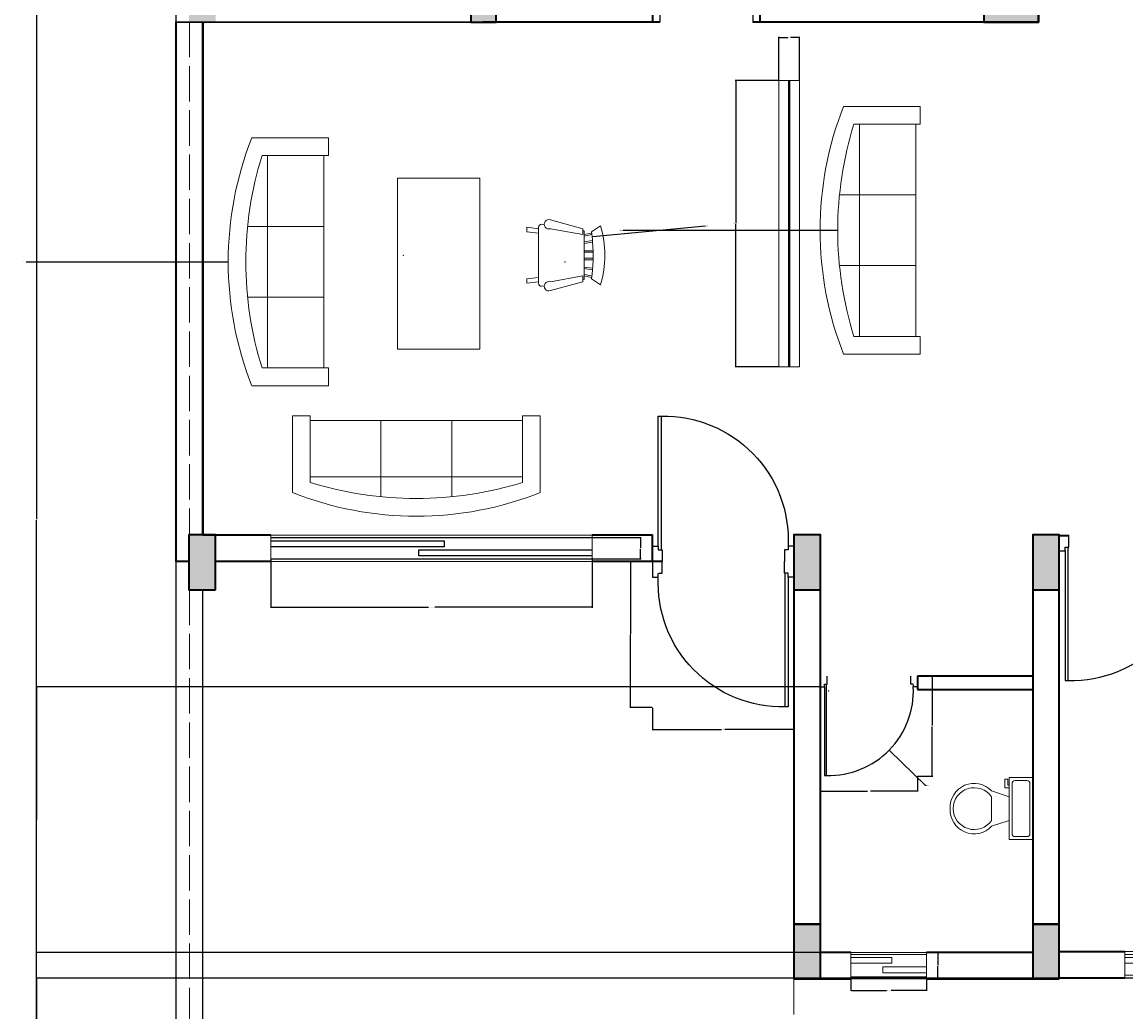
# Model space of a CAD drawing. Units: inches. Extents: x 2711 to 4246, y 540 to 1583.
# Tile 2 of 7: x 2711 to 3086, y 894 to 1230. Entities that reach past the tile are written whole.
import ezdxf

# ---------------------------------------------------------------- set-up
doc = ezdxf.new("R2010")
doc.units = ezdxf.units.IN
doc.linetypes.add('ACAD_ISO02W100', pattern=[15, 12, -3])
for name, color, linetype, lineweight in [('A-ANNO-DIMS', 2, 'Continuous', 18), ('A-COLS', 210, 'Continuous', 35), ('A-COLS-PATT', 6, 'Continuous', 13), ('A-FLOR-FIXT', 112, 'Continuous', 18), ('A-FLOR-OVHD', 225, 'ACAD_ISO02W100', 13), ('A-GLAZ', 4, 'Continuous', 18), ('A-WALL', 1, 'Continuous', 35), ('C-PROP-HIDN', 7, 'ACAD_ISO02W100', 13), ('C-PROP-WALL', 7, 'Continuous', 25), ('DOOR', 32, 'Continuous', 25), ('FURN', 30, 'Continuous', 18)]:
    doc.layers.add(name, color=color, linetype=linetype, lineweight=lineweight)
doc.layers.add('DARK', color=5, linetype='Continuous')
doc.styles.get("Standard").update_dxf_attribs({"font": 'arial.ttf'})
doc.dimstyles.get("Standard").update_dxf_attribs({"dimtxt": 0.18, "dimasz": 0.18, "dimexe": 0.18, "dimexo": 0.0625, "dimgap": 0.09, "dimtad": 0, "dimtih": 1, "dimtoh": 1, "dimdec": 4, "dimzin": 0, "dimdsep": 46, "dimtxsty": 'Standard', "dimcen": 0.09, "dimadec": 0, "dimazin": 0, "dimtfac": 1, "dimtdec": 4, "dimtofl": 0, "dimtmove": 0, "dimatfit": 3, "dimfxl": 1, "dimtolj": 1, "dimtzin": 0, "dimarcsym": 0})

# ---------------------------------------------------------------- blocks, each defined once
blk = doc.blocks.new('DOORS')
at = {"layer": 'DOOR'}
for p, q in [((-0.63, -0.36), (-0.63, -5.61)), ((2.62, -4.36), (2.62, -0.36)), ((44.12, -4.36), (44.12, -0.36)), ((47.37, -0.36), (47.37, -5.61)), ((-0.63, -5.61), (1.37, -5.61)), ((1.37, -5.61), (1.37, -4.36)), ((1.37, -4.36), (2.62, -4.36)), ((1.37, -5.61), (1.37, -49.61)), ((2.37, -49.61), (2.37, -4.36)), ((45.37, -4.36), (44.12, -4.36)), ((47.37, -5.61), (45.37, -5.61)), ((1.37, -49.61), (2.37, -49.61))]:
    blk.add_line(p, q, dxfattribs=at)
for centre, radius, start, end in [((3.41, -7.61), 42.01, 268.5852, 2.7319), ((38.76, -4.99), 6.64, 354.6023, 5.3977)]:
    blk.add_arc(centre, radius, start, end, dxfattribs=at)
blk = doc.blocks.new('DIPDASS')
at = {"layer": 'DARK'}
for p, q in [((0, 0), (109.02, 0)), ((0, -7.25), (109.02, -7.25))]:
    blk.add_line(p, q, dxfattribs=at)
at = {"layer": 'DOOR'}
for points in [[(0, -1.16), (56.28, -1.16), (58.81, -1.16), (58.81, -3.16), (56.28, -3.16), (0, -3.16)], [(109.02, -6.2), (52.74, -6.2), (50.21, -6.2), (50.21, -4.2), (52.74, -4.2), (109.02, -4.2)]]:
    blk.add_lwpolyline(points, dxfattribs=at)
blk = doc.blocks.new('Sofa - Roundback 7 ft.')
for p, q in [((-12.00002, -32.4421), (-12.00003, -6.5971)), ((11.99997, -32.4421), (11.99998, -6.5971)), ((-36.000027, -34), (-36.000027, -11.4696)), ((-35.999844, -13.3819), (35.9998, -13.3819)), ((35.99998, -34), (35.99998, -11.4696)), ((-36.000027, -32.4421), (35.99998, -32.4421))]:
    blk.add_line(p, q)
for points in [[(-36.000027, -34), (-42.000027, -34), (-42.000027, -8)], [(41.99998, -8), (41.99998, -34), (35.99998, -34)]]:
    blk.add_lwpolyline(points)
for centre, radius, start, end in [((0, -114.25), 114.25, 68.43141, 111.5686), ((-0.00001, -127.1968), 121.1968, 72.72033, 107.2797)]:
    blk.add_arc(centre, radius, start, end)
blk = doc.blocks.new('Chair - Rocking')
for p, q in [((-8, -4.5), (-10, -1.5)), ((8, -4.5), (10, -1.5)), ((-8.23428, -6.99939), (-8.3093, -7.47958)), ((-8.23041, -7), (8.23915, -7)), ((-7.5, -4.5), (-7, -7)), ((-6.5, -7), (-7.02225, -4.43)), ((-4.5, -7), (-4.96674, -4.19951)), ((-4, -7), (-4.40532, -4.16272)), ((-1.5, -4.05012), (-1.5, -7)), ((-1, -7), (-1, -4.05012)), ((1, -7), (1, -4.04655)), ((1.5, -4.05012), (1.5, -7)), ((4, -7), (4.40187, -4.18694)), ((4.5, -7), (4.96761, -4.19437)), ((6.5, -7), (7, -4.4057)), ((7.5, -4.5), (7, -7)), ((8.31071, -7.48854), (8.23449, -7.00073)), ((-9, -7.5), (-12, -18.49999)), ((-7, -7.5), (-9, -7.5)), ((-9, -18.49999), (-7, -7.5)), ((7, -7.5), (9, -7.5)), ((9, -18.49999), (7, -7.5)), ((9, -7.5), (12, -18.49999)), ((-10.36644, -20.64523), (-10.5, -21.49999)), ((10.5, -21.49999), (10.3575, -20.58798)), ((-9, -22.49999), (-9.5, -26.49999)), ((0, -22.49999), (-9.5, -22.49999)), ((-8, -26.49999), (-7.5, -22.49999)), ((0, -22.49999), (9.5, -22.49999)), ((8, -26.49999), (7.5, -22.49999)), ((9, -22.49999), (9.5, -26.49999)), ((-9.5, -26.49999), (-8, -26.49999)), ((9.5, -26.49999), (8, -26.49999))]:
    blk.add_line(p, q)
for centre, radius, start, end in [((0, -34.08333), 34.08333, 72.93847, 107.0615), ((0, -68.25004), 64.25, 93.92211, 97.15267), ((0, -68.25004), 64.25, 82.84733, 93.92211), ((-10.5, -18.99999), 1.58114, 161.5651, 18.43495), ((10.5, -18.99999), 1.58114, 161.5651, 18.43495), ((-9.5, -21.49999), 1, 180, 270), ((9.5, -21.49999), 1, 270, 0)]:
    blk.add_arc(centre, radius, start, end)
blk = doc.blocks.new('*U44')
for p, q in [((9.5, -6), (9.5, -2)), ((-10, -8.5), (-8, -8.5)), ((-10, -9.5), (-10, -8.5)), ((-7, -9.5), (-10, -9.5)), ((-8, -8.5), (-8, -8)), ((-7, -8), (-7, -9.5)), ((-4, -8), (-6, -14)), ((4, -8), (6, -14)), ((4, -14), (-4, -14))]:
    blk.add_line(p, q)
blk.add_lwpolyline([(10.5, -8), (10.5, 0), (-10.5, 0), (-10.5, -8)], close=True)
for points in [[(-9.5, -2), (-9.5, -6)], [(8.5, -1), (-8.5, -1)], [(-8.5, -7), (8.5, -7)]]:
    blk.add_lwpolyline(points)
for centre, radius, start, end in [((-8.625, -1.875), 0.8839, 81.8699, 188.1301), ((8.625, -1.875), 0.8839, 351.8699, 98.1301), ((-8.625, -6.125), 0.8839, 171.869898, 278.1301), ((8.625, -6.125), 0.8839, 261.8699, 8.1301), ((-0.4772, -19.9188), 8.0953, 133.01722, 273.38), ((0.0374, -19.8731), 7.127, 124.50543, 269.7), ((-0.0373, -19.8731), 7.127, 270.3, 55.4946), ((0.4773, -19.9188), 8.0953, 266.62, 46.9828)]:
    blk.add_arc(centre, radius, start, end)
blk = doc.blocks.new('SCREEN-LIVING')
for p, q in [((0, 97.11), (0, 0)), ((7, 97.11), (0, 97.11)), ((3.25, 97.11), (3.25, 0)), ((3.5, 97.11), (3.5, 0)), ((3.75, 97.11), (3.75, 0)), ((7, 0), (7, 97.11)), ((0, 0), (7, 0))]:
    blk.add_line(p, q)
blk = doc.blocks.new('WIN-SLIDER-W02')
for p, q in [((0, 9), (0, 0)), ((0, 9), (25.68, 9)), ((0, 8.3), (25.68, 8.3)), ((25.68, 9), (25.68, 0)), ((0, 7.32), (13.85, 7.32)), ((13.85, 5.32), (0, 5.32)), ((10.83, 2.09), (10.83, 4.09)), ((10.83, 4.09), (25.68, 4.09)), ((13.85, 7.32), (13.85, 5.32)), ((0, 0.7), (25.68, 0.7)), ((25.68, 2.09), (10.83, 2.09)), ((0, 0), (25.68, 0))]:
    blk.add_line(p, q)
blk = doc.blocks.new('WIN-SLIDER-W03')
for p, q in [((0, 9), (0, 0)), ((99.07, 9), (0, 9)), ((0, 8.03), (99.07, 8.03)), ((99.07, 9), (99.07, 0)), ((0, 7.05), (54.2, 7.05)), ((54.2, 5.05), (0, 5.05)), ((45.64, 1.82), (45.64, 3.82)), ((45.64, 3.82), (99.07, 3.82)), ((54.2, 7.05), (54.2, 5.05)), ((0, 0.97), (99.07, 0.97)), ((99.07, 1.82), (45.64, 1.82)), ((0, 0), (99.07, 0))]:
    blk.add_line(p, q)
blk = doc.blocks.new('*D56')
at = {"layer": 'A-ANNO-DIMS', "color": 0, "lineweight": -2, "transparency": 16777216}
for p, q in [((2924.96, 1047.04), (2917.41, 1047.04)), ((2917.59, 1046.86), (2917.59, 1022.45)), ((2917.59, 997.68), (2917.59, 1022.09)), ((2924.96, 997.5), (2917.41, 997.5))]:
    blk.add_line(p, q, dxfattribs=at)
at = {"layer": 'A-ANNO-DIMS', "color": 0, "transparency": 16777216}
for points in [[(2917.56, 1046.86), (2917.62, 1046.86), (2917.59, 1047.04)], [(2917.56, 997.68), (2917.62, 997.68), (2917.59, 997.5)]]:
    blk.add_solid(points, dxfattribs=at)
at = {"layer": 'Defpoints', "color": 0, "transparency": 16777216}
for p in [(2917.59, 1047.04), (2925.02, 1047.04), (2925.02, 997.5)]:
    blk.add_point(p, dxfattribs=at)
at = {"layer": 'A-ANNO-DIMS', "color": 0, "transparency": 16777216, "insert": (2917.59, 1022.27), "char_height": 0.18, "attachment_point": 5}
blk.add_mtext('\\A1;DOOR 50 TYP.', dxfattribs=at)
blk = doc.blocks.new('*D57')
at = {"layer": 'A-ANNO-DIMS', "color": 0, "lineweight": -2, "transparency": 16777216}
for p, q in [((2925.02, 997.44), (2925.02, 989.89)), ((2973.02, 997.44), (2973.02, 989.89)), ((2925.2, 990.07), (2948.49, 990.07)), ((2972.84, 990.07), (2949.55, 990.07))]:
    blk.add_line(p, q, dxfattribs=at)
at = {"layer": 'A-ANNO-DIMS', "color": 0, "transparency": 16777216}
for points in [[(2925.2, 990.1), (2925.2, 990.04), (2925.02, 990.07)], [(2972.84, 990.1), (2972.84, 990.04), (2973.02, 990.07)]]:
    blk.add_solid(points, dxfattribs=at)
at = {"layer": 'Defpoints', "color": 0, "transparency": 16777216}
for p in [(2925.02, 997.5), (2973.02, 997.5), (2925.02, 990.07)]:
    blk.add_point(p, dxfattribs=at)
at = {"layer": 'A-ANNO-DIMS', "color": 0, "transparency": 16777216, "insert": (2949.02, 990.07), "char_height": 0.18, "attachment_point": 5}
blk.add_mtext('\\A1;48 TYP.', dxfattribs=at)
blk = doc.blocks.new('*D58')
at = {"layer": 'A-ANNO-DIMS', "color": 0, "lineweight": -2, "transparency": 16777216}
for p, q in [((3014.93, 1008.16), (3020.13, 1008.16)), ((3019.95, 1007.98), (3019.95, 991.4)), ((3019.95, 974.46), (3019.95, 991.03)), ((3014.93, 974.28), (3020.13, 974.28))]:
    blk.add_line(p, q, dxfattribs=at)
at = {"layer": 'A-ANNO-DIMS', "color": 0, "transparency": 16777216}
for points in [[(3019.92, 1007.98), (3019.98, 1007.98), (3019.95, 1008.16)], [(3019.92, 974.46), (3019.98, 974.46), (3019.95, 974.28)]]:
    blk.add_solid(points, dxfattribs=at)
at = {"layer": 'Defpoints', "color": 0, "transparency": 16777216}
for p in [(3014.87, 1008.16), (3019.95, 1008.16), (3014.87, 974.28)]:
    blk.add_point(p, dxfattribs=at)
at = {"layer": 'A-ANNO-DIMS', "color": 0, "transparency": 16777216, "insert": (3019.95, 991.22), "char_height": 0.18, "attachment_point": 5}
blk.add_mtext('\\A1;DOOR 34 TYP.', dxfattribs=at)
blk = doc.blocks.new('*D59')
at = {"layer": 'A-ANNO-DIMS', "color": 0, "lineweight": -2, "transparency": 16777216}
for p, q in [((2982.04, 974.22), (2982.04, 969.02)), ((3014.87, 974.22), (3014.87, 969.02)), ((2982.22, 969.2), (2997.93, 969.2)), ((3014.69, 969.2), (2998.98, 969.2))]:
    blk.add_line(p, q, dxfattribs=at)
at = {"layer": 'A-ANNO-DIMS', "color": 0, "transparency": 16777216}
for points in [[(2982.22, 969.23), (2982.22, 969.17), (2982.04, 969.2)], [(3014.69, 969.23), (3014.69, 969.17), (3014.87, 969.2)]]:
    blk.add_solid(points, dxfattribs=at)
at = {"layer": 'Defpoints', "color": 0, "transparency": 16777216}
for p in [(2982.04, 974.28), (3014.87, 974.28), (3014.87, 969.2)]:
    blk.add_point(p, dxfattribs=at)
at = {"layer": 'A-ANNO-DIMS', "color": 0, "transparency": 16777216, "insert": (2998.45, 969.2), "char_height": 0.18, "attachment_point": 5}
blk.add_mtext('\\A1;33 TYP.', dxfattribs=at)
blk = doc.blocks.new('*D62')
at = {"layer": 'A-ANNO-DIMS', "color": 0, "lineweight": -2, "transparency": 16777216}
for p, q in [((2795.61, 1047.85), (2795.61, 1031.38)), ((2904.63, 1047.85), (2904.63, 1031.38)), ((2795.79, 1031.56), (2849.03, 1031.56)), ((2904.45, 1031.56), (2851.21, 1031.56))]:
    blk.add_line(p, q, dxfattribs=at)
at = {"layer": 'A-ANNO-DIMS', "color": 0, "transparency": 16777216}
for points in [[(2795.79, 1031.59), (2795.79, 1031.53), (2795.61, 1031.56)], [(2904.45, 1031.59), (2904.45, 1031.53), (2904.63, 1031.56)]]:
    blk.add_solid(points, dxfattribs=at)
at = {"layer": 'Defpoints', "color": 0, "transparency": 16777216}
for p in [(2795.61, 1047.91), (2904.63, 1047.91), (2904.63, 1031.56)]:
    blk.add_point(p, dxfattribs=at)
at = {"layer": 'A-ANNO-DIMS', "color": 0, "transparency": 16777216, "insert": (2850.12, 1031.56), "char_height": 0.18, "attachment_point": 5}
blk.add_mtext('\\A1;SLIDER 109 TYP.', dxfattribs=at)
blk = doc.blocks.new('*D63')
at = {"layer": 'A-ANNO-DIMS', "color": 0, "lineweight": -2, "transparency": 16777216}
for p, q in [((2904.69, 1055.17), (2921.16, 1055.17)), ((2920.98, 1054.99), (2920.98, 1051.72)), ((2920.98, 1048.09), (2920.98, 1051.36)), ((2904.69, 1047.91), (2921.16, 1047.91))]:
    blk.add_line(p, q, dxfattribs=at)
at = {"layer": 'A-ANNO-DIMS', "color": 0, "transparency": 16777216}
for points in [[(2920.95, 1054.99), (2921.01, 1054.99), (2920.98, 1055.17)], [(2920.95, 1048.09), (2921.01, 1048.09), (2920.98, 1047.91)]]:
    blk.add_solid(points, dxfattribs=at)
at = {"layer": 'Defpoints', "color": 0, "transparency": 16777216}
for p in [(2904.63, 1055.17), (2920.98, 1055.17), (2904.63, 1047.91)]:
    blk.add_point(p, dxfattribs=at)
at = {"layer": 'A-ANNO-DIMS', "color": 0, "transparency": 16777216, "insert": (2920.98, 1051.54), "char_height": 0.18, "attachment_point": 5}
blk.add_mtext('\\A1;7 TYP.', dxfattribs=at)
blk = doc.blocks.new('*D84')
at = {"layer": 'A-ANNO-DIMS', "color": 0, "lineweight": -2, "transparency": 16777216}
for p, q in [((2967.8, 1210.19), (2953.12, 1210.19)), ((2953.3, 1210.01), (2953.3, 1161.81)), ((2953.3, 1113.26), (2953.3, 1161.45)), ((2967.8, 1113.08), (2953.12, 1113.08))]:
    blk.add_line(p, q, dxfattribs=at)
at = {"layer": 'A-ANNO-DIMS', "color": 0, "transparency": 16777216}
for points in [[(2953.27, 1210.01), (2953.33, 1210.01), (2953.3, 1210.19)], [(2953.27, 1113.26), (2953.33, 1113.26), (2953.3, 1113.08)]]:
    blk.add_solid(points, dxfattribs=at)
at = {"layer": 'Defpoints', "color": 0, "transparency": 16777216}
for p in [(2953.3, 1210.19), (2967.87, 1210.19), (2967.87, 1113.08)]:
    blk.add_point(p, dxfattribs=at)
at = {"layer": 'A-ANNO-DIMS', "color": 0, "transparency": 16777216, "insert": (2953.3, 1161.63), "char_height": 0.18, "attachment_point": 5}
blk.add_mtext('\\A1;SCREEN 97 TYP.', dxfattribs=at)
blk = doc.blocks.new('*D85')
at = {"layer": 'A-ANNO-DIMS', "color": 0, "lineweight": -2, "transparency": 16777216}
for p, q in [((2967.87, 1210.25), (2967.87, 1224.93)), ((2968.05, 1224.75), (2970.91, 1224.75)), ((2974.69, 1224.75), (2971.82, 1224.75)), ((2974.87, 1210.25), (2974.87, 1224.93))]:
    blk.add_line(p, q, dxfattribs=at)
at = {"layer": 'A-ANNO-DIMS', "color": 0, "transparency": 16777216}
for points in [[(2968.05, 1224.78), (2968.05, 1224.72), (2967.87, 1224.75)], [(2974.69, 1224.78), (2974.69, 1224.72), (2974.87, 1224.75)]]:
    blk.add_solid(points, dxfattribs=at)
at = {"layer": 'Defpoints', "color": 0, "transparency": 16777216}
for p in [(2974.87, 1224.75), (2967.87, 1210.19), (2974.87, 1210.19)]:
    blk.add_point(p, dxfattribs=at)
at = {"layer": 'A-ANNO-DIMS', "color": 0, "transparency": 16777216, "insert": (2971.37, 1224.75), "char_height": 0.18, "attachment_point": 5}
blk.add_mtext('\\A1;7 TYP.', dxfattribs=at)
blk = doc.blocks.new('*D88')
at = {"layer": 'A-ANNO-DIMS', "color": 0, "lineweight": -2, "transparency": 16777216}
for p, q in [((2992.34, 905.43), (2992.34, 901.46)), ((3018.02, 905.43), (3018.02, 901.46)), ((2992.52, 901.64), (3004.36, 901.64)), ((3017.84, 901.64), (3006.01, 901.64))]:
    blk.add_line(p, q, dxfattribs=at)
at = {"layer": 'A-ANNO-DIMS', "color": 0, "transparency": 16777216}
for points in [[(2992.52, 901.67), (2992.52, 901.61), (2992.34, 901.64)], [(3017.84, 901.67), (3017.84, 901.61), (3018.02, 901.64)]]:
    blk.add_solid(points, dxfattribs=at)
at = {"layer": 'Defpoints', "color": 0, "transparency": 16777216}
for p in [(2992.34, 905.5), (3018.02, 905.5), (3018.02, 901.64)]:
    blk.add_point(p, dxfattribs=at)
at = {"layer": 'A-ANNO-DIMS', "color": 0, "transparency": 16777216, "insert": (3005.18, 901.64), "char_height": 0.18, "attachment_point": 5}
blk.add_mtext('\\A1;W02 26 TYP.', dxfattribs=at)
blk = doc.blocks.new('*D89')
at = {"layer": 'A-ANNO-DIMS', "color": 0, "lineweight": -2, "transparency": 16777216}
for p, q in [((3018.08, 914.5), (3022.05, 914.5)), ((3021.87, 914.32), (3021.87, 910.18)), ((3021.87, 905.68), (3021.87, 909.81)), ((3018.08, 905.5), (3022.05, 905.5))]:
    blk.add_line(p, q, dxfattribs=at)
at = {"layer": 'A-ANNO-DIMS', "color": 0, "transparency": 16777216}
for points in [[(3021.84, 914.32), (3021.9, 914.32), (3021.87, 914.5)], [(3021.84, 905.68), (3021.9, 905.68), (3021.87, 905.5)]]:
    blk.add_solid(points, dxfattribs=at)
at = {"layer": 'Defpoints', "color": 0, "transparency": 16777216}
for p in [(3018.02, 914.5), (3021.87, 914.5), (3018.02, 905.5)]:
    blk.add_point(p, dxfattribs=at)
at = {"layer": 'A-ANNO-DIMS', "color": 0, "transparency": 16777216, "insert": (3021.87, 910), "char_height": 0.18, "attachment_point": 5}
blk.add_mtext('\\A1;9 TYP.', dxfattribs=at)
blk = doc.blocks.new('*D95')
at = {"layer": 'A-ANNO-DIMS', "color": 0, "lineweight": -2, "transparency": 16777216}
for p, q in [((2763.43, 1534.95), (2715.94, 1534.95)), ((2716.12, 1534.77), (2716.12, 1061.38)), ((2716.12, 587.63), (2716.12, 1061.02)), ((2763.43, 587.45), (2715.94, 587.45))]:
    blk.add_line(p, q, dxfattribs=at)
at = {"layer": 'A-ANNO-DIMS', "color": 0, "transparency": 16777216}
for points in [[(2716.09, 1534.77), (2716.15, 1534.77), (2716.12, 1534.95)], [(2716.09, 587.63), (2716.15, 587.63), (2716.12, 587.45)]]:
    blk.add_solid(points, dxfattribs=at)
at = {"layer": 'Defpoints', "color": 0, "transparency": 16777216}
for p in [(2716.12, 1534.95), (2763.5, 1534.95), (2763.5, 587.45)]:
    blk.add_point(p, dxfattribs=at)
at = {"layer": 'A-ANNO-DIMS', "color": 0, "transparency": 16777216, "insert": (2716.12, 1061.2), "char_height": 0.18, "attachment_point": 5}
blk.add_mtext('\\A1;947.5', dxfattribs=at)
blk = doc.blocks.new('*D104')
at = {"layer": 'A-ANNO-DIMS', "color": 0, "lineweight": -2, "transparency": 16777216}
for p, q in [((3215.96, 905.77), (2715.94, 905.77)), ((2716.12, 905.59), (2716.12, 865.45)), ((2716.12, 824.95), (2716.12, 865.09)), ((3215.96, 824.77), (2715.94, 824.77))]:
    blk.add_line(p, q, dxfattribs=at)
at = {"layer": 'A-ANNO-DIMS', "color": 0, "transparency": 16777216}
for points in [[(2716.09, 905.59), (2716.15, 905.59), (2716.12, 905.77)], [(2716.09, 824.95), (2716.15, 824.95), (2716.12, 824.77)]]:
    blk.add_solid(points, dxfattribs=at)
at = {"layer": 'Defpoints', "color": 0, "transparency": 16777216}
for p in [(3216.02, 905.77), (2716.12, 824.77), (3216.02, 824.77)]:
    blk.add_point(p, dxfattribs=at)
at = {"layer": 'A-ANNO-DIMS', "color": 0, "transparency": 16777216, "insert": (2716.12, 865.27), "char_height": 0.18, "attachment_point": 5}
blk.add_mtext('\\A1;81', dxfattribs=at)
blk = doc.blocks.new('*D115')
at = {"layer": 'A-ANNO-DIMS', "color": 0, "lineweight": -2, "transparency": 16777216}
for p, q in [((2981.98, 1004.57), (2715.94, 1004.57)), ((2716.12, 1004.39), (2716.12, 959.71)), ((2716.12, 914.68), (2716.12, 959.35)), ((2981.96, 914.5), (2715.94, 914.5))]:
    blk.add_line(p, q, dxfattribs=at)
at = {"layer": 'A-ANNO-DIMS', "color": 0, "transparency": 16777216}
for points in [[(2716.09, 1004.39), (2716.15, 1004.39), (2716.12, 1004.57)], [(2716.09, 914.68), (2716.15, 914.68), (2716.12, 914.5)]]:
    blk.add_solid(points, dxfattribs=at)
at = {"layer": 'Defpoints', "color": 0, "transparency": 16777216}
for p in [(2716.12, 1004.57), (2982.04, 1004.57), (2982.02, 914.5)]:
    blk.add_point(p, dxfattribs=at)
at = {"layer": 'A-ANNO-DIMS', "color": 0, "transparency": 16777216, "insert": (2716.12, 959.53), "char_height": 0.18, "attachment_point": 5}
blk.add_mtext('\\A1;90.07', dxfattribs=at)
blk = doc.blocks.new('*D126')
at = {"layer": 'A-ANNO-DIMS', "color": 0, "lineweight": -2, "transparency": 16777216}
for p, q in [((2915.15, 1159.36), (2987.69, 1159.36)), ((3108.98, 1159.36), (3109.16, 1159.36)), ((3109.07, 1159.27), (3109.07, 1159.45))]:
    blk.add_line(p, q, dxfattribs=at)
at = {"layer": 'A-ANNO-DIMS', "color": 0, "transparency": 16777216}
blk.add_solid([(2987.69, 1159.39), (2987.69, 1159.33), (2987.87, 1159.36)], dxfattribs=at)
at = {"layer": 'Defpoints', "color": 0, "transparency": 16777216}
for p in [(2987.87, 1159.36), (3109.07, 1159.36)]:
    blk.add_point(p, dxfattribs=at)
at = {"layer": 'A-ANNO-DIMS', "color": 0, "transparency": 16777216, "insert": (2914.48, 1159.36), "char_height": 0.18, "attachment_point": 5}
blk.add_mtext('\\A1;3X R121.2', dxfattribs=at)
blk = doc.blocks.new('*D127')
at = {"layer": 'A-ANNO-DIMS', "color": 0, "lineweight": -2, "transparency": 16777216}
for p, q in [((2712.59, 1148.67), (2780.96, 1148.67)), ((2895.3, 1148.67), (2895.48, 1148.67)), ((2895.39, 1148.58), (2895.39, 1148.76))]:
    blk.add_line(p, q, dxfattribs=at)
at = {"layer": 'A-ANNO-DIMS', "color": 0, "transparency": 16777216}
blk.add_solid([(2780.96, 1148.7), (2780.96, 1148.64), (2781.14, 1148.67)], dxfattribs=at)
at = {"layer": 'Defpoints', "color": 0, "transparency": 16777216}
for p in [(2781.14, 1148.67), (2895.39, 1148.67)]:
    blk.add_point(p, dxfattribs=at)
at = {"layer": 'A-ANNO-DIMS', "color": 0, "transparency": 16777216, "insert": (2711.85, 1148.67), "char_height": 0.18, "attachment_point": 5}
blk.add_mtext('\\A1;3X R114.25', dxfattribs=at)
blk = doc.blocks.new('*D128')
at = {"layer": 'A-ANNO-DIMS', "color": 0, "lineweight": -2, "transparency": 16777216}
for p, q in [((2942.97, 1160.8), (2904.78, 1157.1)), ((2840.56, 1150.88), (2840.74, 1150.88)), ((2840.65, 1150.79), (2840.65, 1150.97))]:
    blk.add_line(p, q, dxfattribs=at)
at = {"layer": 'A-ANNO-DIMS', "color": 0, "transparency": 16777216}
blk.add_solid([(2904.78, 1157.13), (2904.78, 1157.07), (2904.6, 1157.08)], dxfattribs=at)
at = {"layer": 'Defpoints', "color": 0, "transparency": 16777216}
for p in [(2904.6, 1157.08), (2840.65, 1150.88)]:
    blk.add_point(p, dxfattribs=at)
at = {"layer": 'A-ANNO-DIMS', "color": 0, "transparency": 16777216, "insert": (2943.65, 1160.8), "char_height": 0.18, "attachment_point": 5}
blk.add_mtext('\\A1;2X R64.25', dxfattribs=at)
blk = doc.blocks.new('*D132')
at = {"layer": 'A-ANNO-DIMS', "color": 0, "lineweight": -2, "transparency": 16777216}
for p, q in [((2984.71, 1003.2), (2984.89, 1003.2)), ((2984.8, 1003.11), (2984.8, 1003.29)), ((3017.68, 971.07), (3005.48, 982.99)), ((3017.86, 971.07), (3017.68, 971.07))]:
    blk.add_line(p, q, dxfattribs=at)
at = {"layer": 'A-ANNO-DIMS', "color": 0, "transparency": 16777216}
blk.add_solid([(3005.5, 983.01), (3005.46, 982.97), (3005.35, 983.12)], dxfattribs=at)
at = {"layer": 'Defpoints', "color": 0, "transparency": 16777216}
for p in [(2984.8, 1003.2), (3005.35, 983.12)]:
    blk.add_point(p, dxfattribs=at)
at = {"layer": 'A-ANNO-DIMS', "color": 0, "transparency": 16777216, "insert": (3018.34, 971.07), "char_height": 0.18, "attachment_point": 5}
blk.add_mtext('\\A1;R28.73', dxfattribs=at)

msp = doc.modelspace()

# ---------------------------------------------------------------- hatches: boundary and pattern name
at = {"layer": 'A-COLS-PATT'}
h = msp.add_hatch(color=256, dxfattribs=at)
h.dxf.hatch_style = 1
h.paths.add_polyline_path([(2767.9955, 1384.9055), (2776.9955, 1384.9055), (2776.9955, 1403.4493), (2767.9955, 1403.4493)])
h.paths.add_polyline_path([(3065.5392, 1394.4493), (3065.5392, 1403.4493), (3046.9955, 1403.4493), (3046.9955, 1394.4493)])
h.paths.add_polyline_path([(3298.9955, 1394.4493), (3298.9955, 1403.4493), (3280.4517, 1403.4493), (3280.4517, 1394.4493)])
h.paths.add_polyline_path([(2767.8485, 1230.0438), (2776.8485, 1230.0353), (2776.8485, 1248.5791), (2767.8485, 1248.5791)])
h.paths.add_polyline_path([(2871.9955, 1229.9493), (2871.9955, 1238.9493), (2863.4422, 1238.9493), (2863.4422, 1229.9531), (2867.4955, 1229.9493)])
h.paths.add_polyline_path([(3055.9955, 1229.9493), (3055.9955, 1238.9493), (3037.4517, 1238.9493), (3037.4517, 1229.9493)])
h.paths.add_polyline_path([(3298.9955, 1229.9493), (3298.9955, 1238.9493), (3280.4517, 1238.9493), (3280.4517, 1229.9493)])
h.paths.add_polyline_path([(2776.8485, 1056.0394), (2767.8485, 1056.0394), (2767.8485, 1037.4957), (2776.8485, 1037.4957)])
h.paths.add_polyline_path([(2973.0214, 1041.7894), (2973.0214, 1037.4957), (2982.0148, 1037.4957), (2982.0148, 1056.0394), (2973.0148, 1056.0394), (2973.0148, 1052.2894), (2973.0214, 1052.2894), (2973.0214, 1047.0394)])
h.paths.add_polyline_path([(3063.0214, 1037.4957), (3063.0214, 1056.0394), (3054.0214, 1056.0394), (3054.0214, 1037.4957)])
h.paths.add_polyline_path([(3294.4955, 1046.9493), (3298.9955, 1046.9493), (3298.9955, 1055.9413), (3280.4517, 1055.9413), (3280.4517, 1046.9493)])
h.paths.add_polyline_path([(2982.0214, 924.0394), (2973.0214, 924.0394), (2973.0214, 905.4957), (2982.0214, 905.4957)])
h.paths.add_polyline_path([(3054.0214, 905.4957), (3063.0214, 905.4957), (3063.0214, 924.0394), (3054.0214, 924.0394)])
h.paths.add_polyline_path([(3216.0214, 905.7675), (3216.0214, 914.7675), (3197.4776, 914.7675), (3197.4776, 905.7675)])
h.paths.add_polyline_path([(2776.8485, 842.8947), (2776.8485, 861.4385), (2767.8485, 861.4385), (2767.8485, 842.8947)])
h.paths.add_polyline_path([(3294.4955, 824.7675), (3298.9955, 824.7498), (3298.9955, 833.7498), (3280.4517, 833.7498), (3280.4517, 824.7675)])
h.paths.add_polyline_path([(2793.6045, 587.4493), (2793.6045, 599.3563), (2767.9955, 599.3563), (2767.9955, 587.4493)])
h.paths.add_polyline_path([(2922.1577, 587.4493), (2922.1577, 596.4493), (2913.6045, 596.4493), (2913.6045, 587.4493)])
h.paths.add_polyline_path([(2995.7668, 587.4493), (2995.7668, 599.3563), (2970.1577, 599.3563), (2970.1577, 587.4493)])

# ---------------------------------------------------------------- linework, layer by layer
at = {"layer": 'A-COLS'}
for points in [[(2863.4422, 1229.9493), (2871.9955, 1229.9493), (2871.9955, 1238.9493), (2863.4422, 1238.9493)], [(3055.9955, 1238.9493), (3037.4517, 1238.9493), (3037.4517, 1229.9493), (3055.9955, 1229.9493)], [(2776.8485, 1037.4957), (2776.8485, 1056.0394), (2767.8485, 1056.0394), (2767.8485, 1037.4957)], [(2982.0148, 1037.4957), (2982.0148, 1056.0394), (2973.0148, 1056.0394), (2973.0148, 1037.4957)], [(3063.0214, 1037.4957), (3063.0214, 1056.0394), (3054.0214, 1056.0394), (3054.0214, 1037.4957)], [(2982.0214, 905.4957), (2982.0214, 924.0394), (2973.0214, 924.0394), (2973.0214, 905.4957)], [(3063.0214, 905.4957), (3063.0214, 924.0394), (3054.0214, 924.0394), (3054.0214, 905.4957)]]:
    msp.add_lwpolyline(points, close=True, dxfattribs=at)
at = {"layer": 'A-FLOR-OVHD'}
msp.add_line((2973.0214, 905.4957), (2973.0214, 844.38), dxfattribs=at)
at = {"layer": 'A-GLAZ'}
for p, q in [((2795.6074, 1056.0394), (2795.6074, 1047.0394)), ((2795.6074, 1056.0217), (2904.6302, 1056.0217)), ((2904.6302, 1056.0394), (2904.6302, 1047.0394)), ((2795.6074, 1047.0572), (2904.6302, 1047.0572))]:
    msp.add_line(p, q, dxfattribs=at)
at = {"layer": 'A-WALL'}
for p, q in [((2925.0214, 1238.9493), (2925.0214, 1229.9493)), ((2961.5467, 1229.9493), (2961.5467, 1238.9493)), ((3055.9955, 1238.9493), (3055.9955, 1229.9493)), ((2763.4955, 1230.048), (2867.4955, 1229.9493)), ((2763.4955, 1047.0394), (2763.4955, 1230.048)), ((2772.4955, 1230.0394), (2772.4955, 1056.0394)), ((2772.4955, 1056.0394), (2772.4955, 1230.0394)), ((2927.4945, 1229.9493), (2867.4955, 1229.9493)), ((3055.9955, 1229.9493), (2959.0737, 1229.9493)), ((2772.4955, 1056.0394), (2795.6074, 1056.0394)), ((2904.6302, 1056.0394), (2925.0214, 1056.0394)), ((2925.0214, 1047.0394), (2925.0214, 1056.0394)), ((3063.0214, 1055.9209), (3066.2714, 1055.9209)), ((2767.8485, 1047.0394), (2763.4955, 1047.0394)), ((2795.6074, 1047.0394), (2776.8485, 1047.0394)), ((2928.2714, 1047.0394), (2904.6302, 1047.0394)), ((2970.5467, 1047.0394), (2970.5402, 1047.0394)), ((2973.0214, 1047.0394), (2973.0214, 924.0394)), ((2982.0214, 924.0394), (2982.0214, 1047.0394)), ((3054.0214, 1047.0394), (3054.0214, 924.0394)), ((3063.0214, 924.0394), (3063.0214, 1047.0394)), ((3054.0214, 1008.1586), (3014.8682, 1008.1586)), ((3014.8682, 1008.1586), (3014.8682, 1003.6586)), ((3014.8682, 1003.6586), (3054.0214, 1003.6586)), ((2973.0214, 924.0394), (2982.0214, 924.0394)), ((2973.0214, 924.0394), (2973.0214, 915.0394)), ((3054.0214, 924.0394), (3063.0214, 924.0394)), ((3063.0214, 915.0394), (3063.0214, 924.0394)), ((2992.3407, 914.4957), (2982.0214, 914.4957)), ((3054.0214, 914.4957), (3018.0214, 914.4957)), ((3063.0214, 914.7675), (3085.2473, 914.7675)), ((3063.0214, 905.7675), (3063.0214, 914.7675)), ((2982.0214, 905.4957), (2992.3407, 905.4957)), ((3018.0214, 905.4957), (3054.0214, 905.4957)), ((3085.2473, 905.7675), (3063.0214, 905.7675))]:
    msp.add_line(p, q, dxfattribs=at)
at = {"layer": 'C-PROP-HIDN'}
for p, q in [((2767.9955, 1230.0353), (2767.9955, 1056.0394)), ((2767.9955, 1037.4957), (2767.9955, 861.4385))]:
    msp.add_line(p, q, dxfattribs=at)
at = {"layer": 'C-PROP-WALL'}
for p, q in [((2763.4955, 587.4493), (2763.4955, 1530.4493)), ((2772.4955, 861.4385), (2772.4955, 1037.4957))]:
    msp.add_line(p, q, dxfattribs=at)
at = {"layer": 'FURN'}
msp.add_lwpolyline([(2838.6037, 1176.9904), (2866.4478, 1176.9904), (2866.4478, 1119.0325), (2838.6037, 1119.0325)], close=True, dxfattribs=at)

# ---------------------------------------------------------------- block references
at = {"layer": 'A-FLOR-FIXT', "rotation": 270}
msp.add_blockref('*U44', (3054.0214, 963.2562), dxfattribs=at)
at = {"layer": 'A-GLAZ'}
for name, p in [('DIPDASS', (2795.6074, 1055.1667)), ('WIN-SLIDER-W02', (2992.341, 905.496)), ('WIN-SLIDER-W03', (3085.247, 905.768))]:
    msp.add_blockref(name, p, dxfattribs=at)
at = {"layer": 'DOOR', "xscale": -0.7609445437706661, "yscale": 0.7609445437706661, "zscale": 0.7609445437706661, "rotation": 180}
msp.add_blockref('DOORS', (2925.4985, 1229.6738), dxfattribs=at)
at = {"layer": 'DOOR', "xscale": -1, "rotation": 180}
msp.add_blockref('DOORS', (2925.6484, 1046.6774), dxfattribs=at)
at = {"layer": 'DOOR'}
msp.add_blockref('DOORS', (3063.6484, 1056.283), dxfattribs=at)
at = {"layer": 'DOOR', "xscale": -1}
msp.add_blockref('DOORS', (2972.3943, 1047.4015), dxfattribs=at)
at = {"layer": 'DOOR', "xscale": 0.6839369753563443, "yscale": 0.6839369753563443, "zscale": 0.6839369753563443}
msp.add_blockref('DOORS', (2982.4681, 1008.4063), dxfattribs=at)
at = {"layer": 'FURN'}
msp.add_blockref('SCREEN-LIVING', (2967.866, 1113.075), dxfattribs=at)
for name, p, rotation in [('Sofa - Roundback 7 ft.', (2981.8717, 1159.3638), 90), ('Sofa - Roundback 7 ft.', (2781.1434, 1148.6686), 90), ('Chair - Rocking', (2908.9012, 1150.8828), 270.0000000000012), ('Sofa - Roundback 7 ft.', (2844.96, 1062.4013), 180)]:
    msp.add_blockref(name, p, dxfattribs=dict(at, rotation=rotation))

# ---------------------------------------------------------------- dimensions: what is measured, and where the dimension line sits
at = {"layer": 'A-ANNO-DIMS'}
for base, p1, p2, override, picture, middle in [((2716.1185, 1534.9493), (2763.4955, 587.4493), (2763.4955, 1534.9493), {"dimdec": 1, "dimlfac": 1, "dimrnd": 0, "dimzin": 0, "dimdsep": 46, "dimlunit": 2}, '*D95', (2716.1185, 1061.1993)), ((2716.1185, 1004.568), (2982.0214, 914.4957), (2982.0393, 1004.568), {"dimdec": 2, "dimlfac": 1, "dimrnd": 0, "dimzin": 0, "dimdsep": 46, "dimlunit": 2}, '*D115', (2716.1185, 959.5318)), ((2716.1185, 824.7675), (3216.0214, 905.7675), (3216.0214, 824.7675), {"dimdec": 0, "dimlfac": 1, "dimrnd": 0, "dimzin": 0, "dimdsep": 46, "dimlunit": 2}, '*D104', (2716.1185, 865.2675))]:
    dim = msp.add_linear_dim(base=base, p1=p1, p2=p2, angle=90, dimstyle='Standard', override=override, dxfattribs=at)
    dim.commit()
    dim.dimension.update_dxf_attribs({"geometry": picture, "text_midpoint": middle})
for base, p1, p2, text, picture, middle in [((2974.8663, 1224.754), (2967.8663, 1210.1872), (2974.8663, 1210.1872), '<> TYP.', '*D85', (2971.3663, 1224.754)), ((2904.6302, 1031.5588), (2795.6074, 1047.9122), (2904.6302, 1047.9122), 'SLIDER <> TYP.', '*D62', (2850.1188, 1031.5588)), ((3014.8682, 969.1955), (2982.0393, 974.2777), (3014.8682, 974.2777), '<> TYP.', '*D59', (2998.4538, 969.1955)), ((3018.0214, 901.6436), (2992.3407, 905.4957), (3018.0214, 905.4957), 'W02 <> TYP.', '*D88', (3005.1811, 901.6436))]:
    dim = msp.add_linear_dim(base=base, p1=p1, p2=p2, text=text, dimstyle='Standard', override={"dimdec": 0, "dimlfac": 1, "dimrnd": 0, "dimzin": 0, "dimdsep": 46, "dimlunit": 2}, dxfattribs=at)
    dim.commit()
    dim.dimension.update_dxf_attribs({"geometry": picture, "text_midpoint": middle})
for base, p1, p2, angle, text, picture, middle in [((2953.2995, 1210.1872), (2967.8663, 1113.0752), (2967.8663, 1210.1872), 90, 'SCREEN <> TYP.', '*D84', (2953.2995, 1161.6312)), ((2920.9836, 1055.1667), (2904.6302, 1047.9122), (2904.6302, 1055.1667), 90, '<> TYP.', '*D63', (2920.9836, 1051.5394)), ((2917.5907, 1047.0394), (2925.0214, 997.5013), (2925.0214, 1047.0394), 90, 'DOOR <> TYP.', '*D56', (2917.5907, 1022.2704)), ((3019.9504, 1008.1586), (3014.8682, 974.2777), (3014.8682, 1008.1586), 90, 'DOOR <> TYP.', '*D58', (3019.9504, 991.2182)), ((2925.0214, 990.0706), (2973.0214, 997.5013), (2925.0214, 997.5013), 180, '<> TYP.', '*D57', (2949.0214, 990.0706)), ((3021.8735, 914.4957), (3018.0214, 905.4957), (3018.0214, 914.4957), 90, '<> TYP.', '*D89', (3021.8735, 909.9957))]:
    dim = msp.add_linear_dim(base=base, p1=p1, p2=p2, angle=angle, text=text, dimstyle='Standard', override={"dimdec": 0, "dimlfac": 1, "dimrnd": 0, "dimzin": 0, "dimdsep": 46, "dimlunit": 2}, dxfattribs=at)
    dim.commit()
    dim.dimension.update_dxf_attribs({"geometry": picture, "text_midpoint": middle})
for center, mpoint, text, override, picture, middle in [((2840.6512, 1150.8828), (2904.6013, 1157.083), '2X <>', {"dimdec": 2, "dimlfac": 1, "dimrnd": 0, "dimzin": 0, "dimdsep": 46, "dimlunit": 2}, '*D128', (2942.9714, 1160.8031)), ((3109.0685, 1159.3638), (2987.8717, 1159.364), '3X <>', {"dimdec": 1, "dimlfac": 1, "dimrnd": 0, "dimzin": 0, "dimdsep": 46, "dimlunit": 2}, '*D126', (2915.1537, 1159.3641)), ((2895.3934, 1148.6686), (2781.1434, 1148.669), '3X <>', {"dimdec": 2, "dimlfac": 1, "dimrnd": 0, "dimzin": 0, "dimdsep": 46, "dimlunit": 2}, '*D127', (2712.5934, 1148.6692))]:
    dim = msp.add_radius_dim(center=center, mpoint=mpoint, text=text, dimstyle='Standard', override=override, dxfattribs=at)
    dim.commit()
    dim.dimension.update_dxf_attribs({"geometry": picture, "text_midpoint": middle, "dimtype": 164})
dim = msp.add_radius_dim(center=(2984.8005, 1003.1985), mpoint=(3005.3496, 983.1164), dimstyle='Standard', override={"dimdec": 2, "dimlfac": 1, "dimrnd": 0, "dimzin": 0, "dimdsep": 46, "dimlunit": 2}, dxfattribs=at)
dim.commit()
dim.dimension.update_dxf_attribs({"geometry": '*D132', "text_midpoint": (3018.3389, 971.0671), "dimtype": 164})

doc.saveas('drawing.dxf')
